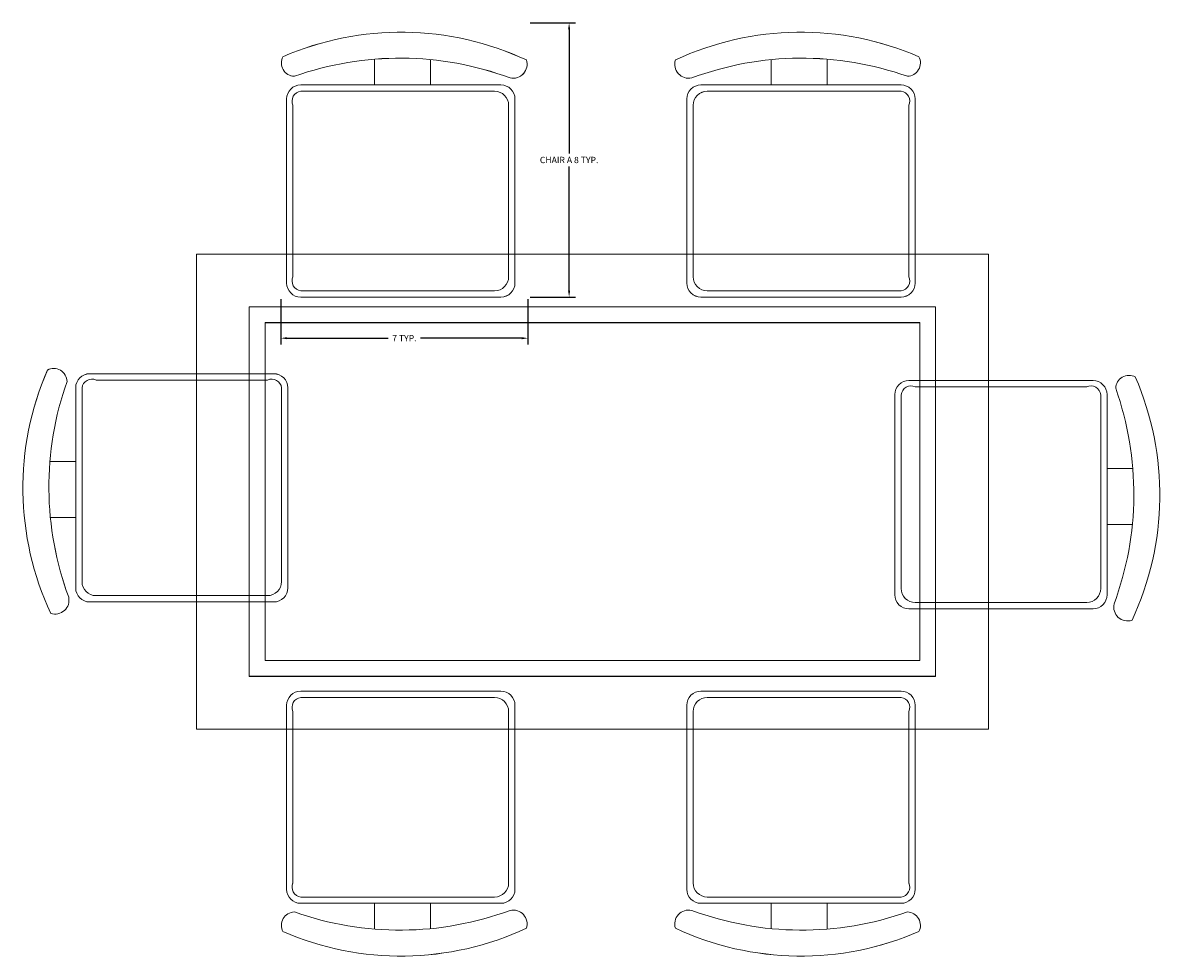
# Model space of a CAD drawing. Units: inches. Extents: x 1962 to 2771, y 1245 to 2660.
# Tile 11 of 114: x 2459 to 2492, y 1734 to 1760. Entities that reach past the tile are written whole.
import ezdxf

# ---------------------------------------------------------------- set-up
doc = ezdxf.new("R2010")
doc.units = ezdxf.units.IN
doc.layers.add('A-ANNO-DIMS', color=2, linetype='Continuous', lineweight=18)
doc.layers.add('A-FURN', color=8, linetype='Continuous', lineweight=13)
doc.styles.get("Standard").update_dxf_attribs({"font": 'arial.ttf'})
doc.dimstyles.get("Standard").update_dxf_attribs({"dimtxt": 0.18, "dimasz": 0.18, "dimexe": 0.18, "dimexo": 0.0625, "dimgap": 0.09, "dimtad": 0, "dimtih": 1, "dimtoh": 1, "dimdec": 4, "dimzin": 0, "dimdsep": 46, "dimtxsty": 'Standard', "dimcen": 0.09, "dimadec": 0, "dimazin": 0, "dimtfac": 1, "dimtdec": 4, "dimtofl": 0, "dimtmove": 0, "dimatfit": 3, "dimfxl": 1, "dimtolj": 1, "dimtzin": 0, "dimarcsym": 0})

# ---------------------------------------------------------------- blocks, each defined once
blk = doc.blocks.new('DINING-TABLE')
for points in [[(0, 13.512), (22.52, 13.512), (22.52, 0), (0, 0)], [(0, 13.512), (22.52, 13.512), (22.52, 0), (0, 0)], [(1.501, 12.011), (21.019, 12.011), (21.019, 1.502), (1.501, 1.502)], [(1.501, 12.011), (21.019, 12.011), (21.019, 1.501), (1.501, 1.501)], [(1.952, 11.561), (20.568, 11.561), (20.568, 1.952), (1.952, 1.952)], [(1.952, 11.56), (20.568, 11.56), (20.568, 1.952), (1.952, 1.952)]]:
    blk.add_lwpolyline(points, close=True)
blk = doc.blocks.new('DINING-CHAIR-A')
for points in [[(0.368, 6.279, -0.175809), (6.502, 6.233, 0.578392), (6.967, 6.744, 0.214524), (0.043, 6.837, 0.552014), (0.368, 6.279, -0.065079)], [(0.368, 6.279, -0.175809), (6.502, 6.232, 0.578392), (6.967, 6.743, 0.214524), (0.043, 6.836, 0.552014), (0.368, 6.279, -0.065079)], [(4.242, 6.033), (4.242, 6.753, -0.064759)], [(4.242, 6.033), (4.242, 6.753, -0.064759)], [(6.242, 6.033), (0.548, 6.033, 0.414214), (0.149, 5.635), (0.149, 0.399, 0.414214), (0.548, 0), (6.242, 0, 0.414214), (6.64, 0.399), (6.64, 5.635, 0.414214), (6.242, 6.033)], [(6.242, 6.033), (0.548, 6.033, 0.414214), (0.149, 5.634), (0.149, 0.398, 0.414214), (0.548, 0), (6.242, 0, 0.414214), (6.641, 0.398), (6.641, 5.634, 0.414214), (6.242, 6.033)]]:
    blk.add_lwpolyline(points, format="xyb")
blk.add_lwpolyline([(2.648, 6.766), (2.648, 6.033)])
blk.add_lwpolyline([(2.648, 6.766), (2.648, 6.033)])
for points in [[(0.55, 5.853), (6.063, 5.853, -0.414214), (6.461, 5.455), (6.461, 0.578, -0.414214), (6.063, 0.18), (0.55, 0.18, -0.512069), (0.329, 0.578), (0.329, 5.455, -0.512069)], [(0.55, 5.853), (6.063, 5.853, -0.414214), (6.461, 5.455), (6.461, 0.578, -0.414214), (6.063, 0.179), (0.55, 0.179, -0.512069), (0.329, 0.578), (0.329, 5.455, -0.512069)]]:
    blk.add_lwpolyline(points, format="xyb", close=True)
blk = doc.blocks.new('DINING-CHAIR-B')
for points in [[(6.279, 6.618, -0.175809), (6.232, 0.484, 0.578392), (6.743, 0.019, 0.214524), (6.836, 6.943, 0.552014), (6.279, 6.618, -0.065079)], [(6.279, 6.618, -0.175809), (6.232, 0.484, 0.578392), (6.743, 0.019, 0.214524), (6.836, 6.943, 0.552014), (6.279, 6.618, -0.065079)], [(6.033, 6.439, 0.414214), (5.634, 6.837), (0.398, 6.837, 0.414214), (0, 6.439), (0, 0.744, 0.414214), (0.398, 0.346), (5.634, 0.346, 0.414214), (6.033, 0.744), (6.033, 6.439)], [(6.033, 6.438, 0.414214), (5.634, 6.837), (0.398, 6.837, 0.414214), (0, 6.438), (0, 0.744, 0.414214), (0.398, 0.346), (5.634, 0.346, 0.414214), (6.033, 0.744), (6.033, 6.438)], [(6.033, 2.744), (6.753, 2.744, -0.064759)], [(6.033, 2.744), (6.753, 2.744, -0.064759)]]:
    blk.add_lwpolyline(points, format="xyb")
for points in [[(5.853, 6.436), (5.853, 0.924, -0.414214), (5.455, 0.525), (0.578, 0.525, -0.414214), (0.179, 0.924), (0.179, 6.436, -0.512069), (0.578, 6.658), (5.455, 6.658, -0.512069)], [(5.853, 6.436), (5.853, 0.923, -0.414214), (5.455, 0.525), (0.578, 0.525, -0.414214), (0.179, 0.923), (0.179, 6.436, -0.512069), (0.578, 6.657), (5.455, 6.657, -0.512069)]]:
    blk.add_lwpolyline(points, format="xyb", close=True)
blk.add_lwpolyline([(6.766, 4.338), (6.033, 4.338)])
blk.add_lwpolyline([(6.766, 4.338), (6.033, 4.338)])
blk = doc.blocks.new('*D34')
at = {"layer": 'A-ANNO-DIMS', "color": 0, "lineweight": -2, "transparency": 16777216}
for p, q in [((2473.557, 1760.149), (2474.845, 1760.149)), ((2474.665, 1759.969), (2474.665, 1756.434)), ((2474.665, 1752.532), (2474.665, 1756.068)), ((2473.557, 1752.352), (2474.845, 1752.352))]:
    blk.add_line(p, q, dxfattribs=at)
at = {"layer": 'A-ANNO-DIMS', "color": 0, "transparency": 16777216}
for points in [[(2474.635, 1759.969), (2474.695, 1759.969), (2474.665, 1760.149)], [(2474.635, 1752.532), (2474.695, 1752.532), (2474.665, 1752.352)]]:
    blk.add_solid(points, dxfattribs=at)
at = {"layer": 'Defpoints', "color": 0, "transparency": 16777216}
for p in [(2473.495, 1760.149), (2474.665, 1760.149), (2473.495, 1752.352)]:
    blk.add_point(p, dxfattribs=at)
at = {"layer": 'A-ANNO-DIMS', "color": 0, "transparency": 16777216, "insert": (2474.665, 1756.251), "char_height": 0.18, "attachment_point": 5}
blk.add_mtext('\\A1;CHAIR A 8 TYP.', dxfattribs=at)
blk = doc.blocks.new('*D35')
at = {"layer": 'A-ANNO-DIMS', "color": 0, "lineweight": -2, "transparency": 16777216}
for p, q in [((2466.467, 1752.29), (2466.467, 1751.002)), ((2473.495, 1752.29), (2473.495, 1751.002)), ((2466.647, 1751.182), (2469.524, 1751.182)), ((2473.315, 1751.182), (2470.438, 1751.182))]:
    blk.add_line(p, q, dxfattribs=at)
at = {"layer": 'A-ANNO-DIMS', "color": 0, "transparency": 16777216}
for points in [[(2466.647, 1751.212), (2466.647, 1751.152), (2466.467, 1751.182)], [(2473.315, 1751.212), (2473.315, 1751.152), (2473.495, 1751.182)]]:
    blk.add_solid(points, dxfattribs=at)
at = {"layer": 'Defpoints', "color": 0, "transparency": 16777216}
for p in [(2466.467, 1752.352), (2473.495, 1752.352), (2473.495, 1751.182)]:
    blk.add_point(p, dxfattribs=at)
at = {"layer": 'A-ANNO-DIMS', "color": 0, "transparency": 16777216, "insert": (2469.981, 1751.182), "char_height": 0.18, "attachment_point": 5}
blk.add_mtext('\\A1;7 TYP.', dxfattribs=at)

msp = doc.modelspace()

# ---------------------------------------------------------------- linework, layer by layer
at = {"layer": 'A-FURN'}
for points in [[(2478.1506, 1758.5848, -0.5783921), (2477.6859, 1759.0957, -0.2145244), (2484.6097, 1759.1886, -0.552014), (2484.2845, 1758.6312, 0.1758092), (2478.1506, 1758.5848)], [(2478.1506, 1758.5845, -0.5783921), (2477.6859, 1759.0955, -0.2145244), (2484.6098, 1759.1884, -0.552014), (2484.2845, 1758.631, 0.1758092), (2478.1506, 1758.5845)], [(2480.411, 1758.385), (2480.411, 1759.1052, 0.0647586)], [(2480.411, 1758.3848), (2480.411, 1759.105, 0.0647586)], [(2484.1053, 1758.385, -0.4142136), (2484.5037, 1757.9867), (2484.5037, 1752.7507, -0.4142136), (2484.1053, 1752.3523), (2478.4108, 1752.3523, -0.4142136), (2478.0124, 1752.7507), (2478.0124, 1757.9867, -0.4142136), (2478.4108, 1758.385), (2484.1053, 1758.385)], [(2484.1053, 1758.3848, -0.4142136), (2484.5037, 1757.9864), (2484.5037, 1752.7505, -0.4142136), (2484.1053, 1752.3521), (2478.4108, 1752.3521, -0.4142136), (2478.0125, 1752.7505), (2478.0125, 1757.9864, -0.4142136), (2478.4108, 1758.3848), (2484.1053, 1758.3848)], [(2460.4356, 1743.8189, -0.5783921), (2459.9247, 1743.3542, -0.2145244), (2459.8318, 1750.278, -0.552014), (2460.3892, 1749.9527, 0.1758094), (2460.4356, 1743.8189)], [(2460.4356, 1743.8186, -0.5783921), (2459.9247, 1743.354, -0.2145244), (2459.8318, 1750.2778, -0.552014), (2460.3892, 1749.9525, 0.1758094), (2460.4356, 1743.8186)], [(2460.6354, 1749.7736, -0.4142136), (2461.0338, 1750.172), (2466.2697, 1750.172, -0.4142136), (2466.6681, 1749.7736), (2466.6681, 1744.0791, -0.4142136), (2466.2697, 1743.6807), (2461.0338, 1743.6807, -0.4142136), (2460.6354, 1744.0791), (2460.6354, 1749.7736)], [(2460.6354, 1749.7734, -0.4142136), (2461.0338, 1750.1717), (2466.2697, 1750.1717, -0.4142136), (2466.6681, 1749.7734), (2466.6681, 1744.0789, -0.4142136), (2466.2697, 1743.6805), (2461.0338, 1743.6805, -0.4142136), (2460.6354, 1744.0789), (2460.6354, 1749.7734)], [(2460.6354, 1746.0793), (2459.9152, 1746.0793, 0.0647586)], [(2460.6354, 1746.0791), (2459.9152, 1746.0791, 0.0647586)], [(2472.7264, 1735.1099), (2467.032, 1735.1099, -0.4142136), (2466.6336, 1735.5083), (2466.6336, 1740.7443, -0.4142136), (2467.032, 1741.1427), (2472.7264, 1741.1427, -0.4142136), (2473.1248, 1740.7443), (2473.1248, 1735.5083, -0.4142136), (2472.7264, 1735.1099)], [(2472.7265, 1735.1097), (2467.032, 1735.1097, -0.4142136), (2466.6336, 1735.5081), (2466.6336, 1740.7441, -0.4142136), (2467.032, 1741.1424), (2472.7265, 1741.1424, -0.4142136), (2473.1249, 1740.7441), (2473.1249, 1735.5081, -0.4142136), (2472.7265, 1735.1097)], [(2484.1053, 1735.1099, 0.4142136), (2484.5037, 1735.5083), (2484.5037, 1740.7443, 0.4142136), (2484.1053, 1741.1427), (2478.4108, 1741.1427, 0.4142136), (2478.0124, 1740.7443), (2478.0124, 1735.5083, 0.4142136), (2478.4108, 1735.1099), (2484.1053, 1735.1099)], [(2484.1053, 1735.1097, 0.4142136), (2484.5037, 1735.5081), (2484.5037, 1740.7441, 0.4142136), (2484.1053, 1741.1424), (2478.4108, 1741.1424, 0.4142136), (2478.0125, 1740.7441), (2478.0125, 1735.5081, 0.4142136), (2478.4108, 1735.1097), (2484.1053, 1735.1097)], [(2470.7263, 1735.1099), (2470.7263, 1734.3898, 0.0647586)], [(2470.7263, 1735.1097), (2470.7263, 1734.3895, 0.0647586)], [(2480.411, 1735.1099), (2480.411, 1734.3898, -0.0647586)], [(2480.411, 1735.1097), (2480.411, 1734.3895, -0.0647586)], [(2472.9867, 1734.9102, -0.5783921), (2473.4514, 1734.3993, -0.2145244), (2466.5275, 1734.3063, -0.552014), (2466.8528, 1734.8638, 0.1758093), (2472.9867, 1734.9102)], [(2472.9867, 1734.91, -0.5783921), (2473.4514, 1734.399, -0.2145244), (2466.5276, 1734.3061, -0.552014), (2466.8528, 1734.8635, 0.1758093), (2472.9867, 1734.91)], [(2484.2845, 1734.8638, -0.1758093), (2478.1506, 1734.9102, 0.5783921), (2477.6859, 1734.3993, 0.2145244), (2484.6097, 1734.3063, 0.552014), (2484.2845, 1734.8638, -0.065079)], [(2484.2845, 1734.8635, -0.1758093), (2478.1506, 1734.91, 0.5783921), (2477.6859, 1734.399, 0.2145244), (2484.6098, 1734.3061, 0.552014), (2484.2845, 1734.8635, -0.065079)]]:
    msp.add_lwpolyline(points, format="xyb", dxfattribs=at)
for points in [[(2482.005, 1759.1183), (2482.005, 1758.385)], [(2482.005, 1759.1181), (2482.005, 1758.3848)], [(2459.9021, 1747.6733), (2460.6354, 1747.6733)], [(2459.9021, 1747.673), (2460.6354, 1747.673)], [(2469.1323, 1734.3767), (2469.1323, 1735.1099)], [(2469.1323, 1734.3764), (2469.1323, 1735.1097)], [(2482.005, 1734.3767), (2482.005, 1735.1099)], [(2482.005, 1734.3764), (2482.005, 1735.1097)]]:
    msp.add_lwpolyline(points, dxfattribs=at)
for points in [[(2484.1029, 1758.2056), (2478.5903, 1758.2056, 0.4142136), (2478.1919, 1757.8072), (2478.1919, 1752.9302, 0.4142136), (2478.5903, 1752.5318), (2484.1029, 1752.5318, 0.5120695), (2484.3242, 1752.9302), (2484.3242, 1757.8072, 0.5120695)], [(2484.1029, 1758.2053), (2478.5903, 1758.2053, 0.4142136), (2478.1919, 1757.8069), (2478.1919, 1752.9299, 0.4142136), (2478.5903, 1752.5315), (2484.1029, 1752.5315, 0.5120695), (2484.3242, 1752.9299), (2484.3242, 1757.8069, 0.5120695)], [(2460.8148, 1749.7712), (2460.8148, 1744.2586, 0.4142136), (2461.2132, 1743.8602), (2466.0902, 1743.8602, 0.4142136), (2466.4886, 1744.2586), (2466.4886, 1749.7712, 0.5120695), (2466.0902, 1749.9925), (2461.2132, 1749.9925, 0.5120695)], [(2460.8148, 1749.7709), (2460.8148, 1744.2584, 0.4142136), (2461.2132, 1743.86), (2466.0902, 1743.86, 0.4142136), (2466.4886, 1744.2584), (2466.4886, 1749.7709, 0.5120695), (2466.0902, 1749.9923), (2461.2132, 1749.9923, 0.5120695)], [(2467.0344, 1735.2894), (2472.547, 1735.2894, 0.4142136), (2472.9454, 1735.6878), (2472.9454, 1740.5648, 0.4142136), (2472.547, 1740.9632), (2467.0344, 1740.9632, 0.5120695), (2466.8131, 1740.5648), (2466.8131, 1735.6878, 0.5120695)], [(2467.0344, 1735.2892), (2472.547, 1735.2892, 0.4142136), (2472.9454, 1735.6876), (2472.9454, 1740.5646, 0.4142136), (2472.547, 1740.963), (2467.0344, 1740.963, 0.5120695), (2466.8131, 1740.5646), (2466.8131, 1735.6876, 0.5120695)], [(2484.1029, 1735.2894), (2478.5903, 1735.2894, -0.4142136), (2478.1919, 1735.6878), (2478.1919, 1740.5648, -0.4142136), (2478.5903, 1740.9632), (2484.1029, 1740.9632, -0.5120695), (2484.3242, 1740.5648), (2484.3242, 1735.6878, -0.5120695)], [(2484.1029, 1735.2892), (2478.5903, 1735.2892, -0.4142136), (2478.1919, 1735.6876), (2478.1919, 1740.5646, -0.4142136), (2478.5903, 1740.963), (2484.1029, 1740.963, -0.5120695), (2484.3242, 1740.5646), (2484.3242, 1735.6876, -0.5120695)]]:
    msp.add_lwpolyline(points, format="xyb", close=True, dxfattribs=at)

# ---------------------------------------------------------------- block references
for name, p in [('DINING-CHAIR-A', (2466.4844, 1752.3521)), ('DINING-TABLE', (2464.0673, 1740.0636)), ('DINING-CHAIR-B', (2483.9265, 1743.1398))]:
    msp.add_blockref(name, p, dxfattribs=at)

# ---------------------------------------------------------------- dimensions: what is measured, and where the dimension line sits
at = {"layer": 'A-ANNO-DIMS'}
dim = msp.add_linear_dim(base=(2474.6646, 1760.1493), p1=(2473.495, 1752.3521), p2=(2473.495, 1760.1493), angle=90, text='CHAIR A <> TYP.', dimstyle='Standard', override={"dimdec": 0, "dimlfac": 1, "dimrnd": 0, "dimzin": 0, "dimdsep": 46, "dimlunit": 2}, dxfattribs=at)
dim.commit()
dim.dimension.update_dxf_attribs({"geometry": '*D34', "text_midpoint": (2474.6646, 1756.2507)})
dim = msp.add_linear_dim(base=(2473.495, 1751.1825), p1=(2466.467, 1752.3521), p2=(2473.495, 1752.3521), text='<> TYP.', dimstyle='Standard', override={"dimdec": 0, "dimlfac": 1, "dimrnd": 0, "dimzin": 0, "dimdsep": 46, "dimlunit": 2}, dxfattribs=at)
dim.commit()
dim.dimension.update_dxf_attribs({"geometry": '*D35', "text_midpoint": (2469.981, 1751.1825)})

doc.saveas('drawing.dxf')
